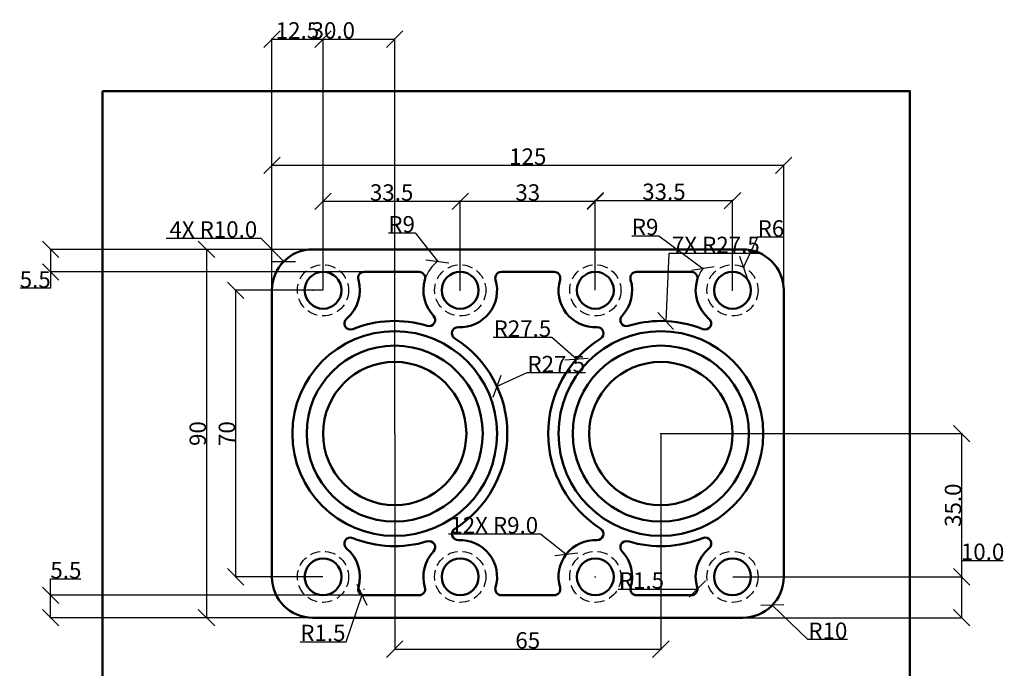
# Model space of a CAD drawing. Units: millimetres. Extents: x 145 to 386, y -112 to 157.
# Tile 2 of 2: x 145 to 386, y -2 to 157. Entities that reach past the tile are written whole.
import ezdxf

# ---------------------------------------------------------------- set-up
doc = ezdxf.new("R2010")
doc.units = ezdxf.units.MM
doc.header["$MEASUREMENT"] = 0
doc.linetypes.add('HIDDEN', pattern=[0.375, 0.25, -0.125])
for name, color, linetype, lineweight in [('M-DIMS', 2, 'Continuous', 25), ('M-HIDN', 8, 'HIDDEN', 25), ('M-OUTL', 7, 'Continuous', 50), ('M-TTLB', 7, 'Continuous', 50)]:
    doc.layers.add(name, color=color, linetype=linetype, lineweight=lineweight)
doc.styles.get("Standard").update_dxf_attribs({"font": 'arial.ttf'})
doc.dimstyles.get("Standard").update_dxf_attribs({"dimtxt": 4, "dimasz": 4, "dimexe": 0.18, "dimexo": 0.0625, "dimgap": 0.09, "dimtad": 1, "dimtoh": 1, "dimdec": 0, "dimzin": 0, "dimdsep": 46, "dimtxsty": 'Standard', "dimblk": 'OBLIQUE', "dimcen": 0.09, "dimclre": 251, "dimadec": 0, "dimazin": 0, "dimtfac": 1, "dimtdec": 0, "dimtofl": 0, "dimtmove": 0, "dimatfit": 3, "dimfxl": 1, "dimtolj": 1, "dimtzin": 0, "dimarcsym": 0})

# ---------------------------------------------------------------- blocks, each defined once
blk = doc.blocks.new('_Oblique')
at = {"color": 0, "linetype": 'ByBlock', "lineweight": -2}
blk.add_line((-0.5, -0.5), (0.5, 0.5), dxfattribs=at)
blk = doc.blocks.new('*D13')
at = {"layer": 'Defpoints', "color": 0, "transparency": 16777216}
for p in [(332.01, 121.11), (207.01, 90.58), (332.01, 90.58)]:
    blk.add_point(p, dxfattribs=at)
at = {"layer": 'M-DIMS', "color": 0, "lineweight": -2, "transparency": 16777216}
for p, q in [((207.01, 90.64), (207.01, 121.29)), ((207.01, 121.11), (332.01, 121.11)), ((332.01, 90.64), (332.01, 121.29))]:
    blk.add_line(p, q, dxfattribs=at)
at = {"layer": 'M-DIMS', "color": 0, "lineweight": -2, "transparency": 16777216, "xscale": 4, "yscale": 4, "zscale": 4, "rotation": 180}
blk.add_blockref('_Oblique', (207.01, 121.11), dxfattribs=at)
at = {"layer": 'M-DIMS', "color": 0, "lineweight": -2, "transparency": 16777216, "xscale": 4, "yscale": 4, "zscale": 4}
blk.add_blockref('_Oblique', (332.01, 121.11), dxfattribs=at)
at = {"layer": 'M-DIMS', "color": 0, "transparency": 16777216, "insert": (269.51, 123.24), "char_height": 4, "attachment_point": 5}
blk.add_mtext('\\A1;125', dxfattribs=at)
blk = doc.blocks.new('*D14')
at = {"layer": 'Defpoints', "color": 0, "transparency": 16777216}
for p in [(253.01, 112.33), (219.51, 90.58), (253.01, 90.58)]:
    blk.add_point(p, dxfattribs=at)
at = {"layer": 'M-DIMS', "color": 0, "lineweight": -2, "transparency": 16777216}
for p, q in [((219.51, 90.64), (219.51, 112.51)), ((219.51, 112.33), (253.01, 112.33)), ((253.01, 90.64), (253.01, 112.51))]:
    blk.add_line(p, q, dxfattribs=at)
at = {"layer": 'M-DIMS', "color": 0, "lineweight": -2, "transparency": 16777216, "xscale": 4, "yscale": 4, "zscale": 4, "rotation": 180}
blk.add_blockref('_Oblique', (219.51, 112.33), dxfattribs=at)
at = {"layer": 'M-DIMS', "color": 0, "lineweight": -2, "transparency": 16777216, "xscale": 4, "yscale": 4, "zscale": 4}
blk.add_blockref('_Oblique', (253.01, 112.33), dxfattribs=at)
at = {"layer": 'M-DIMS', "color": 0, "transparency": 16777216, "insert": (236.26, 114.47), "char_height": 4, "attachment_point": 5}
blk.add_mtext('\\A1;33.5', dxfattribs=at)
blk = doc.blocks.new('*D15')
at = {"layer": 'Defpoints', "color": 0, "transparency": 16777216}
for p in [(286.01, 112.33), (253.01, 90.58), (286.01, 90.58)]:
    blk.add_point(p, dxfattribs=at)
at = {"layer": 'M-DIMS', "color": 0, "lineweight": -2, "transparency": 16777216}
for p, q in [((253.01, 90.64), (253.01, 112.51)), ((253.01, 112.33), (286.01, 112.33)), ((286.01, 90.64), (286.01, 112.51))]:
    blk.add_line(p, q, dxfattribs=at)
at = {"layer": 'M-DIMS', "color": 0, "lineweight": -2, "transparency": 16777216, "xscale": 4, "yscale": 4, "zscale": 4, "rotation": 180}
blk.add_blockref('_Oblique', (253.01, 112.33), dxfattribs=at)
at = {"layer": 'M-DIMS', "color": 0, "lineweight": -2, "transparency": 16777216, "xscale": 4, "yscale": 4, "zscale": 4}
blk.add_blockref('_Oblique', (286.01, 112.33), dxfattribs=at)
at = {"layer": 'M-DIMS', "color": 0, "transparency": 16777216, "insert": (269.51, 114.47), "char_height": 4, "attachment_point": 5}
blk.add_mtext('\\A1;33', dxfattribs=at)
blk = doc.blocks.new('*D16')
at = {"layer": 'Defpoints', "color": 0, "transparency": 16777216}
for p in [(319.51, 112.51), (286.01, 90.58), (319.51, 90.58)]:
    blk.add_point(p, dxfattribs=at)
at = {"layer": 'M-DIMS', "color": 0, "lineweight": -2, "transparency": 16777216}
for p, q in [((286.01, 90.64), (286.01, 112.69)), ((286.01, 112.51), (319.51, 112.51)), ((319.51, 90.64), (319.51, 112.69))]:
    blk.add_line(p, q, dxfattribs=at)
at = {"layer": 'M-DIMS', "color": 0, "lineweight": -2, "transparency": 16777216, "xscale": 4, "yscale": 4, "zscale": 4, "rotation": 180}
blk.add_blockref('_Oblique', (286.01, 112.51), dxfattribs=at)
at = {"layer": 'M-DIMS', "color": 0, "lineweight": -2, "transparency": 16777216, "xscale": 4, "yscale": 4, "zscale": 4}
blk.add_blockref('_Oblique', (319.51, 112.51), dxfattribs=at)
at = {"layer": 'M-DIMS', "color": 0, "transparency": 16777216, "insert": (302.76, 114.65), "char_height": 4, "attachment_point": 5}
blk.add_mtext('\\A1;33.5', dxfattribs=at)
blk = doc.blocks.new('*D17')
at = {"layer": 'Defpoints', "color": 0, "transparency": 16777216}
for p in [(216.95, 100.58), (191.04, 10.58), (216.95, 10.58)]:
    blk.add_point(p, dxfattribs=at)
at = {"layer": 'M-DIMS', "color": 0, "lineweight": -2, "transparency": 16777216}
for p, q in [((216.89, 100.58), (190.86, 100.58)), ((191.04, 100.58), (191.04, 10.58)), ((216.89, 10.58), (190.86, 10.58))]:
    blk.add_line(p, q, dxfattribs=at)
at = {"layer": 'M-DIMS', "color": 0, "lineweight": -2, "transparency": 16777216, "xscale": 4, "yscale": 4, "zscale": 4}
for p, rotation in [((191.04, 100.58), 90), ((191.04, 10.58), 270)]:
    blk.add_blockref('_Oblique', p, dxfattribs=dict(at, rotation=rotation))
at = {"layer": 'M-DIMS', "color": 0, "transparency": 16777216, "insert": (188.91, 55.58), "char_height": 4, "attachment_point": 5, "rotation": 90}
blk.add_mtext('\\A1;90', dxfattribs=at)
blk = doc.blocks.new('*D18')
at = {"layer": 'Defpoints', "color": 0, "transparency": 16777216}
for p in [(219.51, 90.58), (198.16, 20.58), (219.51, 20.58)]:
    blk.add_point(p, dxfattribs=at)
at = {"layer": 'M-DIMS', "color": 0, "lineweight": -2, "transparency": 16777216}
for p, q in [((219.44, 90.58), (197.98, 90.58)), ((198.16, 90.58), (198.16, 20.58)), ((219.44, 20.58), (197.98, 20.58))]:
    blk.add_line(p, q, dxfattribs=at)
at = {"layer": 'M-DIMS', "color": 0, "lineweight": -2, "transparency": 16777216, "xscale": 4, "yscale": 4, "zscale": 4}
for p, rotation in [((198.16, 90.58), 90), ((198.16, 20.58), 270)]:
    blk.add_blockref('_Oblique', p, dxfattribs=dict(at, rotation=rotation))
at = {"layer": 'M-DIMS', "color": 0, "transparency": 16777216, "insert": (196.03, 55.58), "char_height": 4, "attachment_point": 5, "rotation": 90}
blk.add_mtext('\\A1;70', dxfattribs=at)
blk = doc.blocks.new('*D19')
at = {"layer": 'Defpoints', "color": 0, "transparency": 16777216}
for p in [(237.01, 55.58), (302.01, 55.58), (302.01, 2.92)]:
    blk.add_point(p, dxfattribs=at)
at = {"layer": 'M-DIMS', "color": 0, "lineweight": -2, "transparency": 16777216}
for p, q in [((237.01, 55.52), (237.01, 2.74)), ((302.01, 55.52), (302.01, 2.74)), ((237.01, 2.92), (302.01, 2.92))]:
    blk.add_line(p, q, dxfattribs=at)
at = {"layer": 'M-DIMS', "color": 0, "lineweight": -2, "transparency": 16777216, "xscale": 4, "yscale": 4, "zscale": 4, "rotation": 180}
blk.add_blockref('_Oblique', (237.01, 2.92), dxfattribs=at)
at = {"layer": 'M-DIMS', "color": 0, "lineweight": -2, "transparency": 16777216, "xscale": 4, "yscale": 4, "zscale": 4}
blk.add_blockref('_Oblique', (302.01, 2.92), dxfattribs=at)
at = {"layer": 'M-DIMS', "color": 0, "transparency": 16777216, "insert": (269.51, 5.06), "char_height": 4, "attachment_point": 5}
blk.add_mtext('\\A1;65', dxfattribs=at)
blk = doc.blocks.new('*D20')
at = {"layer": 'Defpoints', "color": 0, "transparency": 16777216}
for p in [(247.45, 97.66), (253.01, 90.58)]:
    blk.add_point(p, dxfattribs=at)
at = {"layer": 'M-DIMS', "color": 0, "lineweight": -2, "transparency": 16777216}
for p, q in [((235.47, 104.58), (242.02, 104.58)), ((242.02, 104.58), (247.45, 97.66)), ((252.92, 90.58), (253.1, 90.58)), ((253.01, 90.49), (253.01, 90.67))]:
    blk.add_line(p, q, dxfattribs=at)
blk.add_arc((253.01, 90.58), 9, 127.0025, 163.0006, dxfattribs=at)
at = {"layer": 'M-DIMS', "color": 0, "lineweight": -2, "transparency": 16777216, "xscale": 4, "yscale": 4, "zscale": 4, "rotation": 308.1483947883997}
blk.add_blockref('_Oblique', (247.45, 97.66), dxfattribs=at)
at = {"layer": 'M-DIMS', "color": 0, "transparency": 16777216, "insert": (238.7, 106.71), "char_height": 4, "attachment_point": 5}
blk.add_mtext('\\A1;R9', dxfattribs=at)
blk = doc.blocks.new('*D21')
at = {"layer": 'Defpoints', "color": 0, "transparency": 16777216}
for p in [(312.27, 95.94), (319.51, 90.58)]:
    blk.add_point(p, dxfattribs=at)
at = {"layer": 'M-DIMS', "color": 0, "lineweight": -2, "transparency": 16777216}
for p, q in [((294.94, 103.91), (301.49, 103.91)), ((301.49, 103.91), (312.27, 95.94)), ((319.42, 90.58), (319.6, 90.58)), ((319.51, 90.49), (319.51, 90.67))]:
    blk.add_line(p, q, dxfattribs=at)
blk.add_arc((319.51, 90.58), 9, 142.3511, 163.0006, dxfattribs=at)
at = {"layer": 'M-DIMS', "color": 0, "lineweight": -2, "transparency": 16777216, "xscale": 4, "yscale": 4, "zscale": 4, "rotation": 323.4969972658792}
blk.add_blockref('_Oblique', (312.27, 95.94), dxfattribs=at)
at = {"layer": 'M-DIMS', "color": 0, "transparency": 16777216, "insert": (298.17, 106.05), "char_height": 4, "attachment_point": 5}
blk.add_mtext('\\A1;R9', dxfattribs=at)
blk = doc.blocks.new('*D22')
at = {"layer": 'Defpoints', "color": 0, "transparency": 16777216}
for p in [(322.16, 96.24), (319.51, 90.58)]:
    blk.add_point(p, dxfattribs=at)
at = {"layer": 'M-DIMS', "color": 0, "lineweight": -2, "transparency": 16777216}
for p, q in [((325.59, 103.56), (322.16, 96.24)), ((332.13, 103.56), (325.59, 103.56)), ((319.42, 90.58), (319.6, 90.58)), ((319.51, 90.49), (319.51, 90.67))]:
    blk.add_line(p, q, dxfattribs=at)
at = {"layer": 'M-DIMS', "color": 0, "lineweight": -2, "transparency": 16777216, "xscale": 4, "yscale": 4, "zscale": 4, "rotation": 244.8864642010597}
blk.add_blockref('_Oblique', (322.16, 96.24), dxfattribs=at)
at = {"layer": 'M-DIMS', "color": 0, "transparency": 16777216, "insert": (328.9, 105.69), "char_height": 4, "attachment_point": 5}
blk.add_mtext('\\A1;R6', dxfattribs=at)
blk = doc.blocks.new('*D23')
at = {"layer": 'Defpoints', "color": 0, "transparency": 16777216}
for p in [(322.01, 20.58), (329.22, 13.65)]:
    blk.add_point(p, dxfattribs=at)
at = {"layer": 'M-DIMS', "color": 0, "lineweight": -2, "transparency": 16777216}
for p, q in [((321.92, 20.58), (322.1, 20.58)), ((322.01, 20.49), (322.01, 20.67)), ((337.93, 5.28), (329.22, 13.65)), ((347.57, 5.28), (337.93, 5.28))]:
    blk.add_line(p, q, dxfattribs=at)
at = {"layer": 'M-DIMS', "color": 0, "lineweight": -2, "transparency": 16777216, "xscale": 4, "yscale": 4, "zscale": 4, "rotation": 136.1517874220567}
blk.add_blockref('_Oblique', (329.22, 13.65), dxfattribs=at)
at = {"layer": 'M-DIMS', "color": 0, "transparency": 16777216, "insert": (342.8, 7.42), "char_height": 4, "attachment_point": 5}
blk.add_mtext('\\A1;R10', dxfattribs=at)
blk = doc.blocks.new('*D24')
at = {"layer": 'Defpoints', "color": 0, "transparency": 16777216}
for p in [(281.4, 73.8), (302.01, 55.58)]:
    blk.add_point(p, dxfattribs=at)
at = {"layer": 'M-DIMS', "color": 0, "lineweight": -2, "transparency": 16777216}
for p, q in [((261.07, 79.09), (275.41, 79.09)), ((275.41, 79.09), (281.4, 73.8)), ((301.92, 55.58), (302.1, 55.58)), ((302.01, 55.49), (302.01, 55.67))]:
    blk.add_line(p, q, dxfattribs=at)
at = {"layer": 'M-DIMS', "color": 0, "lineweight": -2, "transparency": 16777216, "xscale": 4, "yscale": 4, "zscale": 4, "rotation": 318.5220611144742}
blk.add_blockref('_Oblique', (281.4, 73.8), dxfattribs=at)
at = {"layer": 'M-DIMS', "color": 0, "transparency": 16777216, "insert": (268.2, 81.23), "char_height": 4, "attachment_point": 5}
blk.add_mtext('\\A1;R27.5', dxfattribs=at)
blk = doc.blocks.new('*D25')
at = {"layer": 'Defpoints', "color": 0, "transparency": 16777216}
for p in [(261.99, 67.08), (237.01, 55.58)]:
    blk.add_point(p, dxfattribs=at)
at = {"layer": 'M-DIMS', "color": 0, "lineweight": -2, "transparency": 16777216}
for p, q in [((269.26, 70.43), (261.99, 67.08)), ((283.59, 70.43), (269.26, 70.43)), ((236.92, 55.58), (237.1, 55.58)), ((237.01, 55.49), (237.01, 55.67))]:
    blk.add_line(p, q, dxfattribs=at)
at = {"layer": 'M-DIMS', "color": 0, "lineweight": -2, "transparency": 16777216, "xscale": 4, "yscale": 4, "zscale": 4, "rotation": 204.7158471989894}
blk.add_blockref('_Oblique', (261.99, 67.08), dxfattribs=at)
at = {"layer": 'M-DIMS', "color": 0, "transparency": 16777216, "insert": (276.47, 72.56), "char_height": 4, "attachment_point": 5}
blk.add_mtext('\\A1;R27.5', dxfattribs=at)
blk = doc.blocks.new('*D26')
at = {"layer": 'Defpoints', "color": 0, "transparency": 16777216}
for p in [(309.45, 17.58), (310.95, 17.58)]:
    blk.add_point(p, dxfattribs=at)
at = {"layer": 'M-DIMS', "color": 0, "lineweight": -2, "transparency": 16777216}
blk.add_line((291.62, 17.58), (310.95, 17.58), dxfattribs=at)
at = {"layer": 'M-DIMS', "color": 0, "lineweight": -2, "transparency": 16777216, "xscale": 4, "yscale": 4, "zscale": 4, "rotation": 1.6284e-12}
blk.add_blockref('_Oblique', (310.95, 17.58), dxfattribs=at)
at = {"layer": 'M-DIMS', "color": 0, "transparency": 16777216, "insert": (297.28, 19.71), "char_height": 4, "attachment_point": 5}
blk.add_mtext('\\A1;R1.5', dxfattribs=at)
blk = doc.blocks.new('*D27')
at = {"layer": 'Defpoints', "color": 0, "transparency": 16777216}
for p in [(237.01, 151.93), (207.01, 90.58), (237.01, 55.58)]:
    blk.add_point(p, dxfattribs=at)
at = {"layer": 'M-DIMS', "color": 251, "lineweight": -2, "transparency": 16777216}
for p, q in [((207.01, 90.64), (207.01, 152.11)), ((237.01, 55.64), (237.01, 152.11))]:
    blk.add_line(p, q, dxfattribs=at)
at = {"layer": 'M-DIMS', "color": 0, "lineweight": -2, "transparency": 16777216}
blk.add_line((207.01, 151.93), (237.01, 151.93), dxfattribs=at)
at = {"layer": 'M-DIMS', "color": 0, "lineweight": -2, "transparency": 16777216, "xscale": 4, "yscale": 4, "zscale": 4, "rotation": 180}
blk.add_blockref('_Oblique', (207.01, 151.93), dxfattribs=at)
at = {"layer": 'M-DIMS', "color": 0, "lineweight": -2, "transparency": 16777216, "xscale": 4, "yscale": 4, "zscale": 4}
blk.add_blockref('_Oblique', (237.01, 151.93), dxfattribs=at)
at = {"layer": 'M-DIMS', "color": 0, "transparency": 16777216, "insert": (222.01, 154.06), "char_height": 4, "attachment_point": 5}
blk.add_mtext('\\A1;30.0', dxfattribs=at)
blk = doc.blocks.new('*D28')
at = {"layer": 'Defpoints', "color": 0, "transparency": 16777216}
for p in [(219.51, 151.93), (207.01, 90.58), (219.51, 90.58)]:
    blk.add_point(p, dxfattribs=at)
at = {"layer": 'M-DIMS', "color": 251, "lineweight": -2, "transparency": 16777216}
for p, q in [((207.01, 90.64), (207.01, 152.11)), ((219.51, 90.64), (219.51, 152.11))]:
    blk.add_line(p, q, dxfattribs=at)
at = {"layer": 'M-DIMS', "color": 0, "lineweight": -2, "transparency": 16777216}
blk.add_line((207.01, 151.93), (219.51, 151.93), dxfattribs=at)
at = {"layer": 'M-DIMS', "color": 0, "lineweight": -2, "transparency": 16777216, "xscale": 4, "yscale": 4, "zscale": 4, "rotation": 180}
blk.add_blockref('_Oblique', (207.01, 151.93), dxfattribs=at)
at = {"layer": 'M-DIMS', "color": 0, "lineweight": -2, "transparency": 16777216, "xscale": 4, "yscale": 4, "zscale": 4}
blk.add_blockref('_Oblique', (219.51, 151.93), dxfattribs=at)
at = {"layer": 'M-DIMS', "color": 0, "transparency": 16777216, "insert": (213.26, 154.06), "char_height": 4, "attachment_point": 5}
blk.add_mtext('\\A1;12.5', dxfattribs=at)
blk = doc.blocks.new('*D29')
at = {"layer": 'Defpoints', "color": 0, "transparency": 16777216}
for p in [(217.01, 100.58), (152.95, 95.08), (229.57, 95.08)]:
    blk.add_point(p, dxfattribs=at)
at = {"layer": 'M-DIMS', "color": 251, "lineweight": -2, "transparency": 16777216}
for p, q in [((216.94, 100.58), (152.77, 100.58)), ((229.51, 95.08), (152.77, 95.08))]:
    blk.add_line(p, q, dxfattribs=at)
at = {"layer": 'M-DIMS', "color": 0, "lineweight": -2, "transparency": 16777216}
for p, q in [((152.95, 100.58), (152.95, 95.08)), ((152.95, 95.08), (152.95, 91.08)), ((152.95, 91.08), (145.55, 91.08))]:
    blk.add_line(p, q, dxfattribs=at)
at = {"layer": 'M-DIMS', "color": 0, "lineweight": -2, "transparency": 16777216, "xscale": 4, "yscale": 4, "zscale": 4}
for p, rotation in [((152.95, 100.58), 90), ((152.95, 95.08), 270)]:
    blk.add_blockref('_Oblique', p, dxfattribs=dict(at, rotation=rotation))
at = {"layer": 'M-DIMS', "color": 0, "transparency": 16777216, "insert": (149.21, 93.21), "char_height": 4, "attachment_point": 5}
blk.add_mtext('\\A1;5.5', dxfattribs=at)
blk = doc.blocks.new('*D30')
at = {"layer": 'Defpoints', "color": 0, "transparency": 16777216}
for p in [(152.95, 16.08), (229.57, 16.08), (217.01, 10.58)]:
    blk.add_point(p, dxfattribs=at)
at = {"layer": 'M-DIMS', "color": 0, "lineweight": -2, "transparency": 16777216}
for p, q in [((152.95, 16.08), (152.95, 20.08)), ((152.95, 20.08), (160.35, 20.08)), ((152.95, 10.58), (152.95, 16.08))]:
    blk.add_line(p, q, dxfattribs=at)
at = {"layer": 'M-DIMS', "color": 251, "lineweight": -2, "transparency": 16777216}
for p, q in [((229.51, 16.08), (152.77, 16.08)), ((216.94, 10.58), (152.77, 10.58))]:
    blk.add_line(p, q, dxfattribs=at)
at = {"layer": 'M-DIMS', "color": 0, "lineweight": -2, "transparency": 16777216, "xscale": 4, "yscale": 4, "zscale": 4}
for p, rotation in [((152.95, 16.08), 90), ((152.95, 10.58), 270)]:
    blk.add_blockref('_Oblique', p, dxfattribs=dict(at, rotation=rotation))
at = {"layer": 'M-DIMS', "color": 0, "transparency": 16777216, "insert": (156.7, 22.21), "char_height": 4, "attachment_point": 5}
blk.add_mtext('\\A1;5.5', dxfattribs=at)
blk = doc.blocks.new('*D31')
at = {"layer": 'Defpoints', "color": 0, "transparency": 16777216}
for p in [(319.51, 20.58), (375.5, 20.58), (322.01, 10.58)]:
    blk.add_point(p, dxfattribs=at)
at = {"layer": 'M-DIMS', "color": 0, "lineweight": -2, "transparency": 16777216}
for p, q in [((375.5, 20.58), (375.5, 24.58)), ((375.5, 24.58), (385.59, 24.58)), ((375.5, 10.58), (375.5, 20.58))]:
    blk.add_line(p, q, dxfattribs=at)
at = {"layer": 'M-DIMS', "color": 251, "lineweight": -2, "transparency": 16777216}
for p, q in [((319.57, 20.58), (375.68, 20.58)), ((322.07, 10.58), (375.68, 10.58))]:
    blk.add_line(p, q, dxfattribs=at)
at = {"layer": 'M-DIMS', "color": 0, "lineweight": -2, "transparency": 16777216, "xscale": 4, "yscale": 4, "zscale": 4}
for p, rotation in [((375.5, 20.58), 90), ((375.5, 10.58), 270)]:
    blk.add_blockref('_Oblique', p, dxfattribs=dict(at, rotation=rotation))
at = {"layer": 'M-DIMS', "color": 0, "transparency": 16777216, "insert": (380.59, 26.71), "char_height": 4, "attachment_point": 5}
blk.add_mtext('\\A1;10.0', dxfattribs=at)
blk = doc.blocks.new('*D32')
at = {"layer": 'Defpoints', "color": 0, "transparency": 16777216}
for p in [(302.01, 55.58), (375.5, 55.58), (319.51, 20.58)]:
    blk.add_point(p, dxfattribs=at)
at = {"layer": 'M-DIMS', "color": 251, "lineweight": -2, "transparency": 16777216}
for p, q in [((302.07, 55.58), (375.68, 55.58)), ((319.57, 20.58), (375.68, 20.58))]:
    blk.add_line(p, q, dxfattribs=at)
at = {"layer": 'M-DIMS', "color": 0, "lineweight": -2, "transparency": 16777216}
blk.add_line((375.5, 20.58), (375.5, 55.58), dxfattribs=at)
at = {"layer": 'M-DIMS', "color": 0, "lineweight": -2, "transparency": 16777216, "xscale": 4, "yscale": 4, "zscale": 4}
for p, rotation in [((375.5, 55.58), 90), ((375.5, 20.58), 270)]:
    blk.add_blockref('_Oblique', p, dxfattribs=dict(at, rotation=rotation))
at = {"layer": 'M-DIMS', "color": 0, "transparency": 16777216, "insert": (373.37, 38.08), "char_height": 4, "attachment_point": 5, "rotation": 90}
blk.add_mtext('\\A1;35.0', dxfattribs=at)
blk = doc.blocks.new('*D34')
at = {"layer": 'Defpoints', "color": 0, "transparency": 16777216}
for p in [(303.22, 83.06), (302.01, 55.58)]:
    blk.add_point(p, dxfattribs=at)
at = {"layer": 'M-DIMS', "color": 0, "lineweight": -2, "transparency": 16777216}
for p, q in [((303.94, 99.54), (303.22, 83.06)), ((326.84, 99.54), (303.94, 99.54))]:
    blk.add_line(p, q, dxfattribs=at)
at = {"layer": 'M-DIMS', "color": 251, "lineweight": -2, "transparency": 16777216}
for p, q in [((301.92, 55.58), (302.1, 55.58)), ((302.01, 55.49), (302.01, 55.67))]:
    blk.add_line(p, q, dxfattribs=at)
at = {"layer": 'M-DIMS', "color": 0, "lineweight": -2, "transparency": 16777216, "xscale": 4, "yscale": 4, "zscale": 4, "rotation": 267.4809202232359}
blk.add_blockref('_Oblique', (303.22, 83.06), dxfattribs=at)
at = {"layer": 'M-DIMS', "color": 0, "transparency": 16777216, "insert": (315.44, 101.67), "char_height": 4, "attachment_point": 5}
blk.add_mtext('\\A1;7X R27.5', dxfattribs=at)
blk = doc.blocks.new('*D35')
at = {"layer": 'Defpoints', "color": 0, "transparency": 16777216}
for p in [(209.94, 97.65), (217.01, 90.58)]:
    blk.add_point(p, dxfattribs=at)
at = {"layer": 'M-DIMS', "color": 0, "lineweight": -2, "transparency": 16777216}
for p, q in [((181.23, 103.31), (204.28, 103.31)), ((204.28, 103.31), (209.94, 97.65))]:
    blk.add_line(p, q, dxfattribs=at)
at = {"layer": 'M-DIMS', "color": 251, "lineweight": -2, "transparency": 16777216}
for p, q in [((216.92, 90.58), (217.1, 90.58)), ((217.01, 90.49), (217.01, 90.67))]:
    blk.add_line(p, q, dxfattribs=at)
at = {"layer": 'M-DIMS', "color": 0, "lineweight": -2, "transparency": 16777216, "xscale": 4, "yscale": 4, "zscale": 4, "rotation": 315.0006401248836}
blk.add_blockref('_Oblique', (209.94, 97.65), dxfattribs=at)
at = {"layer": 'M-DIMS', "color": 0, "transparency": 16777216, "insert": (192.71, 105.44), "char_height": 4, "attachment_point": 5}
blk.add_mtext('\\A1;4X R10.0', dxfattribs=at)
blk = doc.blocks.new('*D36')
at = {"layer": 'Defpoints', "color": 0, "transparency": 16777216}
for p in [(278.92, 26.13), (286.01, 20.58)]:
    blk.add_point(p, dxfattribs=at)
at = {"layer": 'M-DIMS', "color": 0, "lineweight": -2, "transparency": 16777216}
for p, q in [((250.11, 31.06), (272.62, 31.06)), ((272.62, 31.06), (278.92, 26.13))]:
    blk.add_line(p, q, dxfattribs=at)
at = {"layer": 'M-DIMS', "color": 251, "lineweight": -2, "transparency": 16777216}
for p, q in [((285.92, 20.58), (286.1, 20.58)), ((286.01, 20.49), (286.01, 20.67))]:
    blk.add_line(p, q, dxfattribs=at)
at = {"layer": 'M-DIMS', "color": 0, "lineweight": -2, "transparency": 16777216, "xscale": 4, "yscale": 4, "zscale": 4, "rotation": 321.9372593833839}
blk.add_blockref('_Oblique', (278.92, 26.13), dxfattribs=at)
at = {"layer": 'M-DIMS', "color": 0, "transparency": 16777216, "insert": (261.32, 33.2), "char_height": 4, "attachment_point": 5}
blk.add_mtext('\\A1;12X R9.0', dxfattribs=at)
blk = doc.blocks.new('*D37')
at = {"layer": 'Defpoints', "color": 0, "transparency": 16777216}
for p in [(229.57, 17.58), (229.08, 16.16)]:
    blk.add_point(p, dxfattribs=at)
at = {"layer": 'M-DIMS', "color": 251, "lineweight": -2, "transparency": 16777216}
for p, q in [((229.48, 17.58), (229.66, 17.58)), ((229.57, 17.49), (229.57, 17.67))]:
    blk.add_line(p, q, dxfattribs=at)
at = {"layer": 'M-DIMS', "color": 0, "lineweight": -2, "transparency": 16777216}
for p, q in [((225.13, 4.74), (229.08, 16.16)), ((213.9, 4.74), (225.13, 4.74))]:
    blk.add_line(p, q, dxfattribs=at)
at = {"layer": 'M-DIMS', "color": 0, "lineweight": -2, "transparency": 16777216, "xscale": 4, "yscale": 4, "zscale": 4, "rotation": 70.9216127119213}
blk.add_blockref('_Oblique', (229.08, 16.16), dxfattribs=at)
at = {"layer": 'M-DIMS', "color": 0, "transparency": 16777216, "insert": (219.47, 6.88), "char_height": 4, "attachment_point": 5}
blk.add_mtext('\\A1;R1.5', dxfattribs=at)

msp = doc.modelspace()

# ---------------------------------------------------------------- linework, layer by layer
at = {"layer": 'M-HIDN', "ltscale": 10}
for centre in [(219.51, 90.58), (253.01, 90.58), (286.01, 90.58), (319.51, 90.58), (219.51, 20.58), (253.01, 20.58), (286.01, 20.58), (319.51, 20.58)]:
    msp.add_circle(centre, 6.25, dxfattribs=at)
at = {"layer": 'M-OUTL'}
for p, q in [((217.01, 100.58), (322.01, 100.58)), ((229.57, 95.08), (242.95, 95.08)), ((263.07, 95.08), (275.95, 95.08)), ((296.07, 95.08), (309.45, 95.08)), ((207.01, 20.58), (207.01, 90.58)), ((332.01, 90.58), (332.01, 20.58)), ((242.95, 16.08), (229.57, 16.08)), ((275.95, 16.08), (263.07, 16.08)), ((309.45, 16.08), (296.07, 16.08)), ((322.01, 10.58), (217.01, 10.58))]:
    msp.add_line(p, q, dxfattribs=at)
for centre, radius in [((219.51, 90.58), 4.5), ((253.01, 90.58), 4.5), ((286.01, 90.58), 4.5), ((319.51, 90.58), 4.5), ((237.01, 55.58), 25), ((302.01, 55.58), 25), ((237.01, 55.58), 21.5), ((302.01, 55.58), 21.5), ((237.01, 55.58), 17.5), ((302.01, 55.58), 17.5), ((219.51, 20.58), 4.5), ((253.01, 20.58), 4.5), ((286.01, 20.58), 4.5), ((319.51, 20.58), 4.5)]:
    msp.add_circle(centre, radius, dxfattribs=at)
for centre, radius, start, end in [((217.01, 90.58), 10, 90, 180), ((322.01, 90.58), 10, 0, 90), ((229.57, 93.58), 1.5, 90, 196.6015), ((242.95, 93.58), 1.5, 343.3985, 90), ((263.07, 93.58), 1.5, 90, 196.6015), ((275.95, 93.58), 1.5, 343.3985, 90), ((296.07, 93.58), 1.5, 90, 196.6015), ((309.45, 93.58), 1.5, 343.3985, 90), ((219.51, 90.58), 9, 309.6249, 16.6015), ((253.01, 90.58), 9, 163.3985, 223.611), ((253.01, 90.58), 9, 267.2546, 16.6015), ((286.01, 90.58), 9, 163.3985, 272.7454), ((286.01, 90.58), 9, 316.389, 16.6015), ((319.51, 90.58), 9, 163.3985, 230.3751), ((245.4, 83.34), 1.5, 253.1677, 43.611), ((293.61, 83.34), 1.5, 136.389, 286.8323), ((226.2, 82.49), 1.5, 129.6249, 291.8721), ((237.01, 55.58), 27.5, 73.1677, 111.8721), ((302.01, 55.58), 27.5, 90, 106.8323), ((302.01, 55.58), 27.5, 68.1279, 90), ((312.81, 82.49), 1.5, 248.1279, 50.3751), ((252.5, 80.09), 1.5, 87.2546, 237.698), ((286.51, 80.09), 1.5, 302.302, 92.7454), ((237.01, 55.58), 27.5, 302.302, 57.698), ((302.01, 55.58), 27.5, 122.302, 237.698), ((252.5, 31.07), 1.5, 122.302, 272.7454), ((286.51, 31.07), 1.5, 267.2546, 57.698), ((226.2, 28.67), 1.5, 68.1279, 230.3751), ((237.01, 55.58), 27.5, 248.1279, 286.8323), ((245.4, 27.82), 1.5, 316.389, 106.8323), ((253.01, 20.58), 9, 343.3985, 92.7454), ((286.01, 20.58), 9, 87.2546, 196.6015), ((293.61, 27.82), 1.5, 73.1677, 223.611), ((302.01, 55.58), 27.5, 253.1677, 291.8721), ((312.81, 28.67), 1.5, 309.6249, 111.8721), ((219.51, 20.58), 9, 343.3985, 50.3751), ((253.01, 20.58), 9, 136.389, 196.6015), ((286.01, 20.58), 9, 343.3985, 43.611), ((319.51, 20.58), 9, 129.6249, 196.6015), ((217.01, 20.58), 10, 180, 270), ((322.01, 20.58), 10, 270, 0), ((229.57, 17.58), 1.5, 163.3985, 270), ((242.95, 17.58), 1.5, 270, 16.6015), ((263.07, 17.58), 1.5, 163.3985, 270), ((275.95, 17.58), 1.5, 270, 16.6015), ((296.07, 17.58), 1.5, 163.3985, 270), ((309.45, 17.58), 1.5, 270, 16.6015)]:
    msp.add_arc(centre, radius, start, end, dxfattribs=at)
at = {"layer": 'M-TTLB'}
msp.add_lwpolyline([(165.63, 139.25), (362.83, 139.25), (362.83, -111.95), (165.63, -111.95)], close=True, dxfattribs=at)

# ---------------------------------------------------------------- dimensions: what is measured, and where the dimension line sits
at = {"layer": 'M-DIMS'}
for base, p1, p2, override, picture, middle in [((237.01, 151.93), (207.01, 90.58), (237.01, 55.58), {"dimdec": 1, "dimlfac": 1, "dimrnd": 0, "dimzin": 0, "dimdsep": 46, "dimlunit": 2}, '*D27', (222.01, 154.06)), ((219.51, 151.93), (207.01, 90.58), (219.51, 90.58), {"dimdec": 1, "dimlfac": 1, "dimrnd": 0, "dimzin": 0, "dimdsep": 46, "dimlunit": 2}, '*D28', (213.26, 154.06)), ((332.01, 121.11), (207.01, 90.58), (332.01, 90.58), {"dimclrd": 0, "dimclre": 0, "dimclrt": 0}, '*D13', (269.51, 123.24)), ((253.01, 112.33), (219.51, 90.58), (253.01, 90.58), {"dimdec": 1, "dimclrd": 0, "dimclre": 0, "dimclrt": 0}, '*D14', (236.26, 114.47)), ((286.01, 112.33), (253.01, 90.58), (286.01, 90.58), {"dimclrd": 0, "dimclre": 0, "dimclrt": 0}, '*D15', (269.51, 114.47)), ((319.51, 112.51), (286.01, 90.58), (319.51, 90.58), {"dimdec": 1, "dimclrd": 0, "dimclre": 0, "dimclrt": 0}, '*D16', (302.76, 114.65)), ((302.01, 2.92), (237.01, 55.58), (302.01, 55.58), {"dimclrd": 0, "dimclre": 0, "dimclrt": 0}, '*D19', (269.51, 5.06))]:
    dim = msp.add_linear_dim(base=base, p1=p1, p2=p2, dimstyle='Standard', override=override, dxfattribs=at)
    dim.commit()
    dim.dimension.update_dxf_attribs({"geometry": picture, "text_midpoint": middle})
for center, mpoint, text, picture, middle in [((217.01, 90.58), (209.94, 97.65), '4X <>', '*D35', (192.71, 105.44)), ((286.01, 20.58), (278.92, 26.13), '12X <>', '*D36', (261.32, 33.2))]:
    dim = msp.add_radius_dim(center=center, mpoint=mpoint, text=text, dimstyle='Standard', override={"dimdec": 1, "dimlfac": 1, "dimrnd": 0, "dimzin": 0, "dimdsep": 46, "dimlunit": 2}, dxfattribs=at)
    dim.commit()
    dim.dimension.update_dxf_attribs({"geometry": picture, "text_midpoint": middle})
for center, mpoint, override, picture, middle in [((253.01, 90.58), (247.45, 97.66), {"dimclrd": 0, "dimclre": 0, "dimclrt": 0}, '*D20', (238.7, 104.58)), ((319.51, 90.58), (312.27, 95.94), {"dimclrd": 0, "dimclre": 0, "dimclrt": 0}, '*D21', (298.17, 103.91)), ((319.51, 90.58), (322.16, 96.24), {"dimclrd": 0, "dimclre": 0, "dimclrt": 0}, '*D22', (328.9, 103.56)), ((309.45, 17.58), (310.95, 17.58), {"dimdec": 1, "dimclrd": 0, "dimclre": 0, "dimclrt": 0}, '*D26', (297.28, 17.58))]:
    dim = msp.add_radius_dim(center=center, mpoint=mpoint, dimstyle='Standard', override=override, dxfattribs=at)
    dim.commit()
    dim.dimension.update_dxf_attribs({"geometry": picture, "text_midpoint": middle, "dimtype": 164})
dim = msp.add_radius_dim(center=(302.01, 55.58), mpoint=(303.22, 83.06), text='7X <>', dimstyle='Standard', override={"dimdec": 1, "dimlfac": 1, "dimrnd": 0, "dimzin": 0, "dimdsep": 46, "dimlunit": 2}, dxfattribs=at)
dim.commit()
dim.dimension.update_dxf_attribs({"geometry": '*D34', "text_midpoint": (315.44, 99.54), "dimtype": 164})
for base, p1, p2, override, picture, middle in [((152.95, 95.08), (217.01, 100.58), (229.57, 95.08), {"dimdec": 1, "dimlfac": 1, "dimrnd": 0, "dimzin": 0, "dimdsep": 46, "dimlunit": 2}, '*D29', (149.21, 93.21)), ((191.04, 10.58), (216.95, 100.58), (216.95, 10.58), {"dimclrd": 0, "dimclre": 0, "dimclrt": 0}, '*D17', (188.91, 55.58)), ((198.16, 20.58), (219.51, 90.58), (219.51, 20.58), {"dimclrd": 0, "dimclre": 0, "dimclrt": 0}, '*D18', (196.03, 55.58)), ((375.5, 55.58), (319.51, 20.58), (302.01, 55.58), {"dimdec": 1, "dimlfac": 1, "dimrnd": 0, "dimzin": 0, "dimdsep": 46, "dimlunit": 2}, '*D32', (373.37, 38.08)), ((375.5, 20.58), (322.01, 10.58), (319.51, 20.58), {"dimdec": 1, "dimlfac": 1, "dimrnd": 0, "dimzin": 0, "dimdsep": 46, "dimlunit": 2}, '*D31', (380.59, 26.71)), ((152.95, 16.08), (217.01, 10.58), (229.57, 16.08), {"dimdec": 1, "dimlfac": 1, "dimrnd": 0, "dimzin": 0, "dimdsep": 46, "dimlunit": 2}, '*D30', (156.7, 22.21))]:
    dim = msp.add_linear_dim(base=base, p1=p1, p2=p2, angle=90, dimstyle='Standard', override=override, dxfattribs=at)
    dim.commit()
    dim.dimension.update_dxf_attribs({"geometry": picture, "text_midpoint": middle})
for center, mpoint, override, picture, middle in [((302.01, 55.58), (281.4, 73.8), {"dimdec": 1, "dimclrd": 0, "dimclre": 0, "dimclrt": 0}, '*D24', (268.2, 81.23)), ((237.01, 55.58), (261.99, 67.08), {"dimdec": 1, "dimclrd": 0, "dimclre": 0, "dimclrt": 0}, '*D25', (276.47, 72.56)), ((322.01, 20.58), (329.22, 13.65), {"dimclrd": 0, "dimclre": 0, "dimclrt": 0}, '*D23', (342.8, 7.42)), ((229.57, 17.58), (229.08, 16.16), {"dimdec": 1, "dimlfac": 1, "dimrnd": 0, "dimzin": 0, "dimdsep": 46, "dimlunit": 2}, '*D37', (219.47, 6.88))]:
    dim = msp.add_radius_dim(center=center, mpoint=mpoint, dimstyle='Standard', override=override, dxfattribs=at)
    dim.commit()
    dim.dimension.update_dxf_attribs({"geometry": picture, "text_midpoint": middle})

doc.saveas('drawing.dxf')
